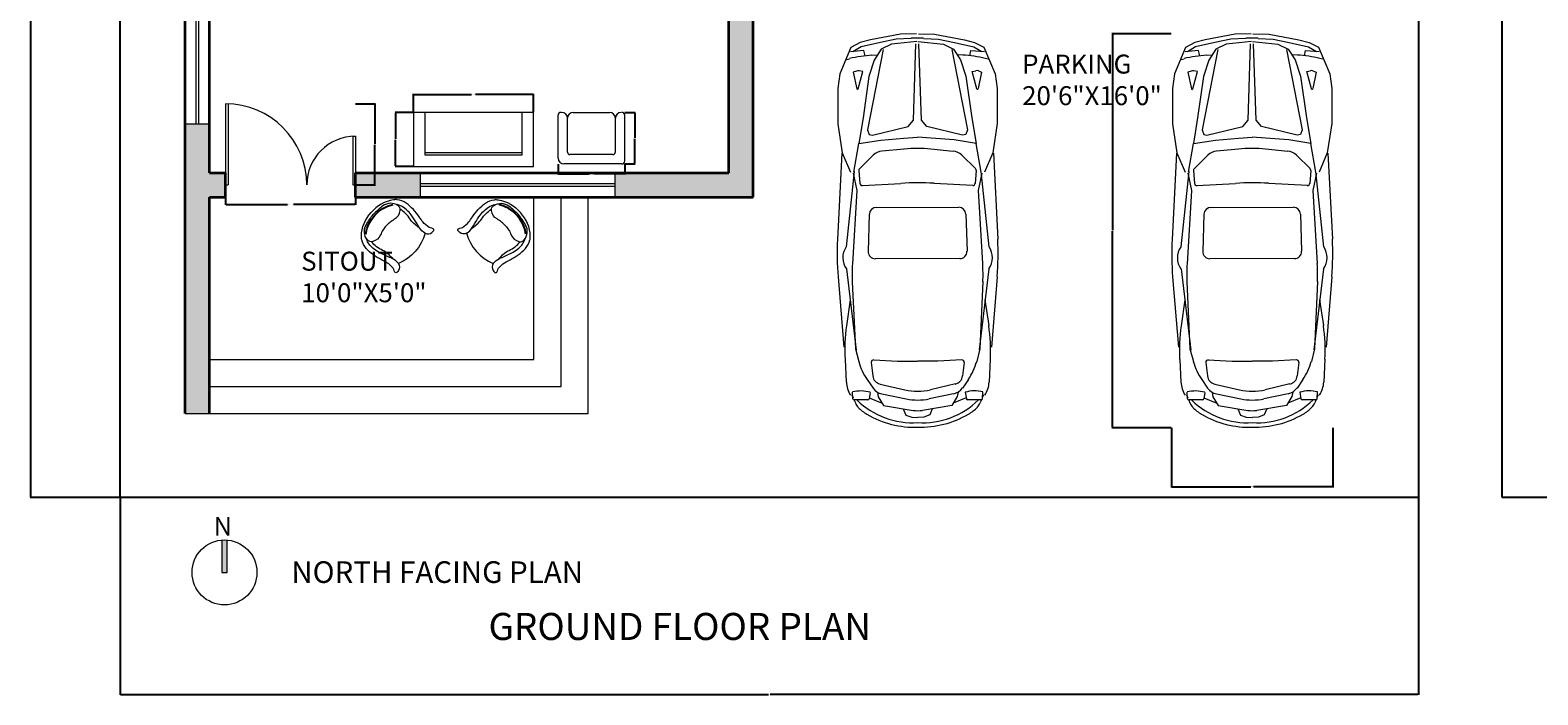
# Model space of a CAD drawing. Units: inches. Extents: x 3386 to 4477, y 1118 to 1824.
# Tile 1 of 7: x 3386 to 3944, y 1118 to 1364. Entities that reach past the tile are written whole.
import ezdxf

# ---------------------------------------------------------------- set-up
doc = ezdxf.new("R2010")
doc.units = ezdxf.units.IN
for name, color, linetype, lineweight in [('A-ANNO-DIMS', 2, 'Continuous', 18), ('A-ANNO-SYMB', 7, 'Continuous', 18), ('A-ANNO-TITL', 7, 'Continuous', 25), ('A-AREA-IDEN', 7, 'Continuous', 18), ('A-DOOR', 4, 'Continuous', 18), ('A-FLOR-STRS', 7, 'Continuous', 18), ('A-FURN', 8, 'Continuous', 18), ('A-GLAZ', 4, 'Continuous', 18), ('A-SITE-VEHI', 8, 'Continuous', 13), ('A-WALL', 7, 'Continuous', 35), ('C-PROP', 7, 'Continuous', 25)]:
    doc.layers.add(name, color=color, linetype=linetype, lineweight=lineweight)
doc.layers.add('A-WALL-PATT', color=18, linetype='Continuous', lineweight=13, true_color=0x000000)
doc.layers.add('IFF-FURN-DETAIL', color=250, linetype='Continuous')
doc.styles.get("Standard").update_dxf_attribs({"font": 'arial.ttf'})
doc.dimstyles.get("Standard").update_dxf_attribs({"dimtxt": 0.18, "dimasz": 0.18, "dimexe": 0.18, "dimexo": 0.0625, "dimgap": 0.09, "dimtad": 0, "dimtih": 1, "dimtoh": 1, "dimdec": 4, "dimzin": 0, "dimdsep": 46, "dimtxsty": 'Standard', "dimcen": 0.09, "dimadec": 0, "dimazin": 0, "dimtfac": 1, "dimtdec": 4, "dimtofl": 0, "dimtmove": 0, "dimatfit": 3, "dimfxl": 1, "dimtolj": 1, "dimtzin": 0, "dimarcsym": 0})

# ---------------------------------------------------------------- blocks, each defined once
blk = doc.blocks.new('D')
for p, q in [((0, 30), (0, 0)), ((1, 29.93), (1, 0)), ((47, 18), (47, 0)), ((47, 18), (48, 18)), ((48, 18), (48, 0)), ((0, 0), (1, 0)), ((47, 0), (48, 0))]:
    blk.add_line(p, q)
for centre, radius, start, end in [((0, 0), 30, 0, 90), ((48, 0), 18, 90, 180)]:
    blk.add_arc(centre, radius, start, end)
blk = doc.blocks.new('sofa-27')
at = {"color": 0, "linetype": 'ByBlock'}
for p, q in [((-0.059, 0.059), (-0.059, 0.49)), ((0.035, 0.118), (0.035, 0.461)), ((0.094, 0.52), (0.459, 0.52)), ((0.518, 0.118), (0.518, 0.461)), ((0.613, 0.03), (0.613, 0.49)), ((0.583, 0), (0, 0)), ((0.494, 0.094), (0.059, 0.094))]:
    blk.add_line(p, q, dxfattribs=at)
for centre, radius, start, end in [((-0.03, 0.49), 0.0295, 90, 180), ((-0.024, 0.461), 0.0591, 360, 90), ((0.094, 0.461), 0.0591, 90, 180), ((0.459, 0.461), 0.0591, 0, 90), ((0.577, 0.461), 0.0591, 90, 180), ((0.583, 0.49), 0.0295, 0, 90), ((0, 0.059), 0.0591, 180, 270), ((0.059, 0.118), 0.0236, 180, 270), ((0.494, 0.118), 0.0236, 270, 0), ((0.583, 0.03), 0.0295, 270, 0)]:
    blk.add_arc(centre, radius, start, end, dxfattribs=at)
blk = doc.blocks.new('12PCOU24')
for p, q in [((9.6, 33.9), (9.6, -34.1)), ((38, 33.9), (38, -34.1))]:
    blk.add_line(p, q)
blk.add_lwpolyline([(0, 42.1), (38, 42.1), (38, 33.9), (8, 33.9), (8, -34.1), (38, -34.1), (38, -42.1), (0, -42.1)], close=True)
blk = doc.blocks.new('A$C4A3239E3')
for p, q in [((1.251, 1.634), (2.152, 1.68)), ((1.443, 1.502), (2.231, 1.588)), ((2.463, 1.587), (3.312, 1.486)), ((2.545, 1.674), (3.282, 1.615)), ((2.788, 1.546), (3.057, 1.586)), ((3.41, 1.602), (3.649, 1.59)), ((0.09, 1.227), (0.136, 1.429)), ((0.136, 1.429), (0.187, 1.515)), ((0.175, 1.399), (0.187, 1.541)), ((0.266, 1.579), (0.259, 1.549)), ((0.396, 1.412), (0.388, 1.449)), ((0.39, 1.477), (0.402, 1.511)), ((0.576, 1.46), (0.396, 1.412)), ((0.402, 1.511), (0.575, 1.474)), ((1.45, 1.506), (1.149, 1.455)), ((1.272, 1.303), (1.413, 1.446)), ((1.433, 1.454), (1.567, 1.444)), ((1.461, 1.515), (1.641, 1.474)), ((1.641, 1.474), (2.408, 1.522)), ((2.597, 1.524), (3.301, 1.494)), ((3.301, 1.494), (3.432, 1.46)), ((3.822, 1.52), (3.752, 1.525)), ((3.781, 1.532), (3.813, 1.518)), ((3.833, 1.363), (3.833, 1.508)), ((3.838, 1.508), (3.867, 1.496)), ((0.231, 1.387), (0.175, 1.399)), ((0.224, 1.314), (0.221, 1.265)), ((1.59, 1.418), (1.567, 1.013)), ((1.819, 0.408), (1.818, 1.271)), ((1.89, 1.345), (2.279, 1.358)), ((2.356, 1.283), (2.357, 0.397)), ((3.416, 1.302), (3.429, 1.052)), ((3.443, 1.328), (3.584, 1.312)), ((3.622, 1.372), (3.711, 1.31)), ((3.753, 1.264), (3.801, 1.255)), ((3.756, 1.339), (3.823, 1.351)), ((3.814, 1.35), (3.869, 1.214)), ((0.056, 1.059), (0.09, 1.227)), ((1.207, 0.98), (1.229, 1.212)), ((3.669, 1.236), (3.73, 0.976)), ((3.771, 1.218), (3.825, 0.963)), ((3.801, 1.255), (3.894, 1.199)), ((3.894, 1.199), (3.945, 0.89)), ((0.048, 0.904), (0.056, 1.059)), ((3.429, 1.052), (3.429, 0.843)), ((3.929, 0.994), (3.993, 0.967)), ((3.993, 0.967), (4.017, 0.906)), ((3.43, 0.631), (3.429, 0.84)), ((3.895, 0.484), (3.945, 0.793)), ((4.017, 0.906), (4.021, 0.842)), ((4.017, 0.778), (4.021, 0.842)), ((0.048, 0.772), (0.057, 0.617)), ((1.208, 0.698), (1.23, 0.466)), ((1.591, 0.261), (1.567, 0.666)), ((3.67, 0.447), (3.73, 0.707)), ((3.772, 0.465), (3.825, 0.721)), ((3.929, 0.689), (3.994, 0.717)), ((3.994, 0.717), (4.017, 0.778)), ((0.057, 0.617), (0.091, 0.45)), ((3.417, 0.38), (3.43, 0.631)), ((3.802, 0.428), (3.895, 0.484)), ((0.091, 0.45), (0.137, 0.247)), ((0.225, 0.362), (0.222, 0.411)), ((1.273, 0.375), (1.415, 0.232)), ((1.891, 0.334), (2.28, 0.323)), ((3.444, 0.354), (3.585, 0.371)), ((3.623, 0.311), (3.712, 0.373)), ((3.754, 0.419), (3.802, 0.428)), ((3.757, 0.344), (3.824, 0.333)), ((3.815, 0.333), (3.869, 0.469)), ((3.834, 0.32), (3.835, 0.175)), ((0.137, 0.247), (0.188, 0.161)), ((0.232, 0.29), (0.176, 0.277)), ((0.176, 0.277), (0.188, 0.136)), ((0.397, 0.265), (0.389, 0.228)), ((0.391, 0.2), (0.403, 0.166)), ((0.577, 0.217), (0.397, 0.265)), ((0.403, 0.166), (0.577, 0.203)), ((1.451, 0.172), (1.15, 0.223)), ((1.434, 0.225), (1.568, 0.235)), ((1.444, 0.176), (2.233, 0.092)), ((1.462, 0.164), (1.642, 0.205)), ((1.642, 0.205), (2.409, 0.158)), ((2.464, 0.094), (3.313, 0.196)), ((2.598, 0.156), (3.302, 0.188)), ((3.302, 0.188), (3.433, 0.223)), ((3.823, 0.163), (3.753, 0.158)), ((3.783, 0.151), (3.814, 0.165)), ((3.839, 0.175), (3.868, 0.188)), ((0.268, 0.097), (0.261, 0.127)), ((1.252, 0.045), (2.154, 0)), ((2.546, 0.006), (3.283, 0.067)), ((2.789, 0.135), (3.058, 0.096)), ((3.412, 0.08), (3.651, 0.093))]:
    blk.add_line(p, q)
for points in [[(0, 0.848), (0.005, 1.016), (0.062, 1.33), (0.09, 1.438), (0.141, 1.536), (0.419, 1.653), (0.572, 1.674), (0.94, 1.674), (1.246, 1.627), (1.45, 1.541)], [(0.081, 0.844), (0.109, 1.11), (0.161, 1.218), (0.274, 1.291), (0.446, 1.347), (0.881, 1.409), (1.149, 1.455), (1.112, 1.224), (1.093, 0.981), (1.085, 0.839)], [(0.164, 1.198), (1.007, 1.364), (1.054, 1.346), (1.062, 1.312), (0.971, 0.937), (0.904, 0.882), (0.106, 0.853)], [(0, 0.828), (0.006, 0.66), (0.063, 0.346), (0.092, 0.239), (0.143, 0.14), (0.42, 0.024), (0.574, 0.003), (0.942, 0.003), (1.247, 0.051), (1.451, 0.138)], [(0.081, 0.832), (0.109, 0.566), (0.162, 0.458), (0.275, 0.386), (0.447, 0.33), (0.882, 0.268), (1.15, 0.223), (1.113, 0.454), (1.094, 0.696), (1.085, 0.839)], [(0.165, 0.478), (1.008, 0.314), (1.055, 0.332), (1.063, 0.366), (0.971, 0.741), (0.904, 0.796), (0.106, 0.823)]]:
    blk.add_lwpolyline(points)
for centre, radius, start, end in [((2.305, -1.296), 2.98, 85.3952, 92.9452), ((2.346, 1.423), 0.202, 54.6492, 124.7769), ((3.317, -0.183), 1.788, 86.9998, 98.3676), ((3.635, 1.312), 0.278, 57.3299, 87.1824), ((1.71, 1.212), 1.49, 166.9166, 176.0811), ((0.436, 1.46), 0.0497, 159.9787, 192.5384), ((0.574, 1.467), 0.00745, 284.96, 78.1125), ((1.431, 1.429), 0.0248, 85.7151, 135.3046), ((1.565, 1.419), 0.0248, 356.7256, 85.7151), ((2.521, -0.262), 1.788, 87.5491, 93.6237), ((3.28, 0.883), 0.596, 55.07, 75.2551), ((4.097, 1.439), 0.356, 166.0961, 196.3535), ((3.821, 1.508), 0.0124, 0, 86.3304), ((3.247, 0.896), 0.828, 356.2451, 44.5195), ((3.809, 1.358), 0.149, 46.3836, 67.2014), ((3.618, 1.158), 0.426, 30.4577, 46.3836), ((1.378, 1.198), 0.149, 135.3046, 174.6214), ((1.892, 1.271), 0.0745, 91.8201, 179.9989), ((2.281, 1.283), 0.0745, 359.9245, 91.8201), ((3.441, 1.304), 0.0248, 83.376, 183.115), ((3.573, 1.213), 0.0993, 13.1226, 83.376), ((3.625, 1.188), 0.149, 11.7694, 55.07), ((3.821, 1.363), 0.0124, 279.6077, 0), ((3.132, 0.872), 0.989, 358.0694, 30.4577), ((2.691, 0.84), 1.49, 174.6214, 185.4916), ((4.542, 0.842), 2.98, 176.7256, 183.3874), ((3.149, 0.841), 0.596, 346.9903, 13.1226), ((3.241, 0.841), 0.596, 348.3436, 11.7694), ((1.238, 0.839), 1.192, 176.8942, 183.2188), ((3.247, 0.786), 0.828, 315.5935, 3.8679), ((3.651, 0.841), 0.298, 350.7246, 9.3883), ((3.133, 0.809), 0.989, 329.6553, 2.0435), ((1.711, 0.467), 1.49, 184.0319, 193.1964), ((1.378, 0.48), 0.149, 185.4916, 224.8083), ((1.893, 0.409), 0.0745, 180.1141, 268.2929), ((2.282, 0.397), 0.0745, 268.2929, 0.1885), ((3.441, 0.379), 0.0248, 176.9979, 276.737), ((3.573, 0.469), 0.0993, 276.737, 346.9903), ((3.626, 0.495), 0.149, 305.0429, 348.3436), ((4.098, 0.244), 0.356, 163.7595, 194.0169), ((3.822, 0.32), 0.0124, 0.113, 80.5053), ((0.438, 0.217), 0.0497, 167.5746, 200.1342), ((0.575, 0.21), 0.00745, 282.0005, 75.153), ((1.432, 0.249), 0.0248, 224.8083, 274.3979), ((1.566, 0.26), 0.0248, 274.3979, 3.3874), ((3.281, 0.799), 0.596, 284.8579, 305.0429), ((3.822, 0.175), 0.0124, 273.7825, 0.113), ((3.81, 0.325), 0.149, 292.9116, 313.7293), ((3.619, 0.525), 0.426, 313.7293, 329.6553), ((2.301, 2.976), 2.98, 267.1678, 274.7177), ((2.347, 0.258), 0.202, 235.336, 305.4638), ((2.518, 1.942), 1.788, 266.4893, 272.5638), ((3.315, 1.865), 1.788, 261.7454, 273.1132), ((3.636, 0.371), 0.278, 272.9306, 302.783)]:
    blk.add_arc(centre, radius, start, end)
blk = doc.blocks.new('ILNG95')
for points in [[(120, 308, -0.32971), (51, 384, -0.036099), (50, 422, -0.497733), (75, 439, -0.070621), (96, 429, 0.101868), (133, 414, 0.091794), (259, 412, 0.024114), (351, 433, -0.090294), (638, 458, -0.132412), (775, 407, -0.068618), (816, 368, -0.184346), (943, 0, 1.803905)], [(120, 308, 0.138132), (244, 313, 0.001085), (325, 339, -0.034227), (462, 375, -0.033255), (567, 387, -0.137428), (727, 350, -4.561553)], [(120, 308, 0.138132), (244, 313, 0.001085), (325, 339, -0.034227), (462, 375, -0.033255), (567, 387, -0.137428), (727, 350, -4.561553)], [(235, 308, 0.064243), (394, 307, 0.04414), (433, 315, -0.118032), (643, 329, -6.296816)], [(235, 308, 0.064243), (394, 307, 0.04414), (433, 315, -0.118032), (643, 329, -6.296816)], [(639, 0, 0.078302), (612, 161, -0.233633), (633, 315, -0.28763), (710, 349, -0.317923), (875, 193, -0.032882), (900, 0, 1.140397)], [(639, 0, 0.078302), (612, 161, -0.233633), (633, 315, -0.28763), (710, 349, -0.317923), (875, 193, -0.032882), (900, 0, 1.140397)], [(120, -308, 0.32971), (51, -384, 0.036099), (50, -422, 0.497733), (75, -439, 0.070621), (96, -429, -0.101868), (133, -414, -0.091794), (259, -412, -0.024114), (351, -433, 0.090294), (638, -458, 0.132412), (775, -407, 0.068618), (816, -368, 0.184346), (943, 0, -1.803905)], [(639, 0, -0.078302), (612, -161, 0.233633), (633, -315, 0.28763), (710, -349, 0.317923), (875, -193, 0.032882), (900, 0, -1.140397)], [(639, 0, -0.078302), (612, -161, 0.233633), (633, -315, 0.28763), (710, -349, 0.317923), (875, -193, 0.032882), (900, 0, -1.140397)], [(120, -308, -0.138132), (244, -313, -0.001085), (325, -339, 0.034227), (462, -375, 0.033255), (567, -387, 0.137428), (727, -350, 4.561553)], [(120, -308, -0.138132), (244, -313, -0.001085), (325, -339, 0.034227), (462, -375, 0.033255), (567, -387, 0.137428), (727, -350, 4.561553)], [(235, -308, -0.064243), (394, -307, -0.04414), (433, -315, 0.118032), (643, -329, 6.296816)], [(235, -308, -0.064243), (394, -307, -0.04414), (433, -315, 0.118032), (643, -329, 6.296816)]]:
    blk.add_lwpolyline(points, format="xyb")
blk.add_arc((759, 1), 709, 154.3281, 205.801)
at = {"layer": 'IFF-FURN-DETAIL'}
blk.add_arc((326, -2), 549, 326.8997, 34.6691, dxfattribs=at)
blk.add_arc((326, -2), 549, 326.8997, 34.6691, dxfattribs=at)
blk = doc.blocks.new('WIN-48IN')
for p, q in [((0, 48), (9, 48)), ((4, 0), (4, 48)), ((5, 0), (5, 48)), ((0, 0), (9, 0))]:
    blk.add_line(p, q)
blk = doc.blocks.new('WIN-72IN')
for p, q in [((0, 0), (0, 9)), ((72, 0), (72, 9)), ((0, 5), (72, 5)), ((0, 4), (72, 4))]:
    blk.add_line(p, q)
blk = doc.blocks.new('NORTH-ARROW')
at = {"transparency": 33554687}
h = blk.add_hatch(color=256, dxfattribs=at)
h.dxf.hatch_style = 1
h.paths.add_polyline_path([(1, 0), (-1, 0), (-1, 11.96, -0.020861), (0, 12, -0.020861), (1, 11.96)])
for p, q in [((-1, 12), (-1, 0)), ((1, 0), (1, 11.96)), ((-1, 0), (1, 0))]:
    blk.add_line(p, q)
blk.add_circle((0, 0), 12)
blk.add_text('N', height=6.9).set_placement((-4.02, 13.6))
blk = doc.blocks.new('*D63')
at = {"layer": 'A-ANNO-DIMS', "color": 0, "lineweight": -2, "transparency": 16777216}
for p, q in [((3458.66, 1306.31), (3458.66, 1298.99)), ((3506.66, 1306.31), (3506.66, 1298.99)), ((3458.84, 1299.17), (3481.57, 1299.17)), ((3506.48, 1299.17), (3483.74, 1299.17))]:
    blk.add_line(p, q, dxfattribs=at)
at = {"layer": 'A-ANNO-DIMS', "color": 0, "transparency": 16777216}
for points in [[(3458.84, 1299.2), (3458.84, 1299.14), (3458.66, 1299.17)], [(3506.48, 1299.2), (3506.48, 1299.14), (3506.66, 1299.17)]]:
    blk.add_solid(points, dxfattribs=at)
at = {"layer": 'Defpoints', "color": 0, "transparency": 16777216}
for p in [(3458.66, 1306.37), (3506.66, 1306.37), (3506.66, 1299.17)]:
    blk.add_point(p, dxfattribs=at)
at = {"layer": 'A-ANNO-DIMS', "color": 0, "transparency": 16777216, "insert": (3482.66, 1299.17), "char_height": 0.18, "attachment_point": 5}
blk.add_mtext('\\A1;ENTRY DOOR 48', dxfattribs=at)
blk = doc.blocks.new('*D64')
at = {"layer": 'A-ANNO-DIMS', "color": 0, "lineweight": -2, "transparency": 16777216}
for p, q in [((3506.72, 1336.37), (3514.04, 1336.37)), ((3513.86, 1336.19), (3513.86, 1321.55)), ((3513.86, 1306.55), (3513.86, 1321.19)), ((3506.72, 1306.37), (3514.04, 1306.37))]:
    blk.add_line(p, q, dxfattribs=at)
at = {"layer": 'A-ANNO-DIMS', "color": 0, "transparency": 16777216}
for points in [[(3513.83, 1336.19), (3513.89, 1336.19), (3513.86, 1336.37)], [(3513.83, 1306.55), (3513.89, 1306.55), (3513.86, 1306.37)]]:
    blk.add_solid(points, dxfattribs=at)
at = {"layer": 'Defpoints', "color": 0, "transparency": 16777216}
for p in [(3506.66, 1336.37), (3513.86, 1336.37), (3506.66, 1306.37)]:
    blk.add_point(p, dxfattribs=at)
at = {"layer": 'A-ANNO-DIMS', "color": 0, "transparency": 16777216, "insert": (3513.86, 1321.37), "char_height": 0.18, "attachment_point": 5}
blk.add_mtext('\\A1;30', dxfattribs=at)
blk = doc.blocks.new('*D71')
at = {"layer": 'A-ANNO-DIMS', "color": 0, "lineweight": -2, "transparency": 16777216}
for p, q in [((3581.59, 1314.07), (3581.59, 1310.26)), ((3581.77, 1310.44), (3593.01, 1310.44)), ((3606.03, 1310.44), (3594.79, 1310.44)), ((3606.21, 1314.07), (3606.21, 1310.26))]:
    blk.add_line(p, q, dxfattribs=at)
at = {"layer": 'A-ANNO-DIMS', "color": 0, "transparency": 16777216}
for points in [[(3581.77, 1310.47), (3581.77, 1310.41), (3581.59, 1310.44)], [(3606.03, 1310.47), (3606.03, 1310.41), (3606.21, 1310.44)]]:
    blk.add_solid(points, dxfattribs=at)
at = {"layer": 'Defpoints', "color": 0, "transparency": 16777216}
for p in [(3581.59, 1314.14), (3606.21, 1314.14), (3606.21, 1310.44)]:
    blk.add_point(p, dxfattribs=at)
at = {"layer": 'A-ANNO-DIMS', "color": 0, "transparency": 16777216, "insert": (3593.9, 1310.44), "char_height": 0.18, "attachment_point": 5}
blk.add_mtext('\\A1;SEAT 25 TYP.', dxfattribs=at)
blk = doc.blocks.new('*D72')
at = {"layer": 'A-ANNO-DIMS', "color": 0, "lineweight": -2, "transparency": 16777216}
for p, q in [((3606.28, 1333.19), (3610.09, 1333.19)), ((3609.91, 1333.01), (3609.91, 1323.85)), ((3609.91, 1314.32), (3609.91, 1323.48)), ((3606.28, 1314.14), (3610.09, 1314.14))]:
    blk.add_line(p, q, dxfattribs=at)
at = {"layer": 'A-ANNO-DIMS', "color": 0, "transparency": 16777216}
for points in [[(3609.88, 1333.01), (3609.94, 1333.01), (3609.91, 1333.19)], [(3609.88, 1314.32), (3609.94, 1314.32), (3609.91, 1314.14)]]:
    blk.add_solid(points, dxfattribs=at)
at = {"layer": 'Defpoints', "color": 0, "transparency": 16777216}
for p in [(3606.21, 1333.19), (3609.91, 1333.19), (3606.21, 1314.14)]:
    blk.add_point(p, dxfattribs=at)
at = {"layer": 'A-ANNO-DIMS', "color": 0, "transparency": 16777216, "insert": (3609.91, 1323.66), "char_height": 0.18, "attachment_point": 5}
blk.add_mtext('\\A1;19 TYP.', dxfattribs=at)
blk = doc.blocks.new('*D85')
at = {"layer": 'A-ANNO-DIMS', "color": 0, "lineweight": -2, "transparency": 16777216}
for p, q in [((3808.27, 1362.25), (3786.31, 1362.25)), ((3786.49, 1362.07), (3786.49, 1289.63)), ((3786.49, 1216.82), (3786.49, 1289.26)), ((3808.27, 1216.64), (3786.31, 1216.64))]:
    blk.add_line(p, q, dxfattribs=at)
at = {"layer": 'A-ANNO-DIMS', "color": 0, "transparency": 16777216}
for points in [[(3786.46, 1362.07), (3786.52, 1362.07), (3786.49, 1362.25)], [(3786.46, 1216.82), (3786.52, 1216.82), (3786.49, 1216.64)]]:
    blk.add_solid(points, dxfattribs=at)
at = {"layer": 'Defpoints', "color": 0, "transparency": 16777216}
for p in [(3808.33, 1362.25), (3786.49, 1216.64), (3808.33, 1216.64)]:
    blk.add_point(p, dxfattribs=at)
at = {"layer": 'A-ANNO-DIMS', "color": 0, "transparency": 16777216, "insert": (3786.49, 1289.45), "char_height": 0.18, "attachment_point": 5}
blk.add_mtext('\\A1;CAR 146 TYP.', dxfattribs=at)
blk = doc.blocks.new('*D86')
at = {"layer": 'A-ANNO-DIMS', "color": 0, "lineweight": -2, "transparency": 16777216}
for p, q in [((3808.33, 1216.58), (3808.33, 1194.62)), ((3868.05, 1216.58), (3868.05, 1194.62)), ((3808.51, 1194.8), (3837.66, 1194.8)), ((3867.87, 1194.8), (3838.72, 1194.8))]:
    blk.add_line(p, q, dxfattribs=at)
at = {"layer": 'A-ANNO-DIMS', "color": 0, "transparency": 16777216}
for points in [[(3808.51, 1194.83), (3808.51, 1194.77), (3808.33, 1194.8)], [(3867.87, 1194.83), (3867.87, 1194.77), (3868.05, 1194.8)]]:
    blk.add_solid(points, dxfattribs=at)
at = {"layer": 'Defpoints', "color": 0, "transparency": 16777216}
for p in [(3808.33, 1216.64), (3868.05, 1216.64), (3868.05, 1194.8)]:
    blk.add_point(p, dxfattribs=at)
at = {"layer": 'A-ANNO-DIMS', "color": 0, "transparency": 16777216, "insert": (3838.19, 1194.8), "char_height": 0.18, "attachment_point": 5}
blk.add_mtext('\\A1;60 TYP.', dxfattribs=at)
blk = doc.blocks.new('*D93')
at = {"layer": 'A-ANNO-DIMS', "color": 0, "lineweight": -2, "transparency": 16777216}
for p, q in [((3528.17, 1333.25), (3528.17, 1340.01)), ((3528.35, 1339.83), (3549.62, 1339.83)), ((3572.27, 1339.83), (3551, 1339.83)), ((3572.45, 1333.25), (3572.45, 1340.01))]:
    blk.add_line(p, q, dxfattribs=at)
at = {"layer": 'A-ANNO-DIMS', "color": 0, "transparency": 16777216}
for points in [[(3528.35, 1339.86), (3528.35, 1339.8), (3528.17, 1339.83)], [(3572.27, 1339.86), (3572.27, 1339.8), (3572.45, 1339.83)]]:
    blk.add_solid(points, dxfattribs=at)
at = {"layer": 'Defpoints', "color": 0, "transparency": 16777216}
for p in [(3572.45, 1339.83), (3528.17, 1333.19), (3572.45, 1333.19)]:
    blk.add_point(p, dxfattribs=at)
at = {"layer": 'A-ANNO-DIMS', "color": 0, "transparency": 16777216, "insert": (3550.31, 1339.83), "char_height": 0.18, "attachment_point": 5}
blk.add_mtext('\\A1;BENCH 44', dxfattribs=at)
blk = doc.blocks.new('*D94')
at = {"layer": 'A-ANNO-DIMS', "color": 0, "lineweight": -2, "transparency": 16777216}
for p, q in [((3528.11, 1333.19), (3521.35, 1333.19)), ((3521.53, 1333.01), (3521.53, 1323.39)), ((3521.53, 1313.4), (3521.53, 1323.02)), ((3528.11, 1313.22), (3521.35, 1313.22))]:
    blk.add_line(p, q, dxfattribs=at)
at = {"layer": 'A-ANNO-DIMS', "color": 0, "transparency": 16777216}
for points in [[(3521.5, 1333.01), (3521.56, 1333.01), (3521.53, 1333.19)], [(3521.5, 1313.4), (3521.56, 1313.4), (3521.53, 1313.22)]]:
    blk.add_solid(points, dxfattribs=at)
at = {"layer": 'Defpoints', "color": 0, "transparency": 16777216}
for p in [(3521.53, 1333.19), (3528.17, 1333.19), (3528.17, 1313.22)]:
    blk.add_point(p, dxfattribs=at)
at = {"layer": 'A-ANNO-DIMS', "color": 0, "transparency": 16777216, "insert": (3521.53, 1323.2), "char_height": 0.18, "attachment_point": 5}
blk.add_mtext('\\A1;20', dxfattribs=at)
blk = doc.blocks.new('*D101')
at = {"layer": 'A-ANNO-DIMS', "color": 0, "lineweight": -2, "transparency": 16777216}
for p, q in [((3419.66, 1190.81), (3419.66, 1117.96)), ((3899.66, 1190.81), (3899.66, 1117.96)), ((3419.84, 1118.14), (3659.36, 1118.14)), ((3899.48, 1118.14), (3659.95, 1118.14))]:
    blk.add_line(p, q, dxfattribs=at)
at = {"layer": 'A-ANNO-DIMS', "color": 0, "transparency": 16777216}
for points in [[(3419.84, 1118.17), (3419.84, 1118.11), (3419.66, 1118.14)], [(3899.48, 1118.17), (3899.48, 1118.11), (3899.66, 1118.14)]]:
    blk.add_solid(points, dxfattribs=at)
at = {"layer": 'Defpoints', "color": 0, "transparency": 16777216}
for p in [(3419.66, 1190.87), (3899.66, 1190.87), (3899.66, 1118.14)]:
    blk.add_point(p, dxfattribs=at)
at = {"layer": 'A-ANNO-DIMS', "color": 0, "transparency": 16777216, "insert": (3659.66, 1118.14), "char_height": 0.18, "attachment_point": 5}
blk.add_mtext('\\A1;480', dxfattribs=at)
blk = doc.blocks.new('*D102')
at = {"layer": 'A-ANNO-DIMS', "color": 0, "lineweight": -2, "transparency": 16777216}
for p, q in [((3419.59, 1790.87), (3386.43, 1790.87)), ((3386.61, 1790.69), (3386.61, 1491.05)), ((3386.61, 1191.05), (3386.61, 1490.69)), ((3419.59, 1190.87), (3386.43, 1190.87))]:
    blk.add_line(p, q, dxfattribs=at)
at = {"layer": 'A-ANNO-DIMS', "color": 0, "transparency": 16777216}
for points in [[(3386.58, 1790.69), (3386.64, 1790.69), (3386.61, 1790.87)], [(3386.58, 1191.05), (3386.64, 1191.05), (3386.61, 1190.87)]]:
    blk.add_solid(points, dxfattribs=at)
at = {"layer": 'Defpoints', "color": 0, "transparency": 16777216}
for p in [(3386.61, 1790.87), (3419.66, 1790.87), (3419.66, 1190.87)]:
    blk.add_point(p, dxfattribs=at)
at = {"layer": 'A-ANNO-DIMS', "color": 0, "transparency": 16777216, "insert": (3386.61, 1490.87), "char_height": 0.18, "attachment_point": 5}
blk.add_mtext('\\A1;600', dxfattribs=at)
blk = doc.blocks.new('*D106')
at = {"layer": 'A-ANNO-DIMS', "color": 0, "lineweight": -2, "transparency": 16777216}
for p, q in [((3963.65, 1790.87), (3930.48, 1790.87)), ((3930.66, 1790.69), (3930.66, 1491.05)), ((3930.66, 1191.05), (3930.66, 1490.69)), ((3963.65, 1190.87), (3930.48, 1190.87))]:
    blk.add_line(p, q, dxfattribs=at)
at = {"layer": 'A-ANNO-DIMS', "color": 0, "transparency": 16777216}
for points in [[(3930.63, 1790.69), (3930.69, 1790.69), (3930.66, 1790.87)], [(3930.63, 1191.05), (3930.69, 1191.05), (3930.66, 1190.87)]]:
    blk.add_solid(points, dxfattribs=at)
at = {"layer": 'Defpoints', "color": 0, "transparency": 16777216}
for p in [(3930.66, 1790.87), (3963.71, 1790.87), (3963.71, 1190.87)]:
    blk.add_point(p, dxfattribs=at)
at = {"layer": 'A-ANNO-DIMS', "color": 0, "transparency": 16777216, "insert": (3930.66, 1490.87), "char_height": 0.18, "attachment_point": 5}
blk.add_mtext('\\A1;600', dxfattribs=at)

msp = doc.modelspace()

# ---------------------------------------------------------------- hatches: boundary and pattern name
at = {"layer": 'A-WALL-PATT'}
h = msp.add_hatch(color=256, dxfattribs=at)
h.dxf.hatch_style = 1
h.paths.add_polyline_path([(3443.66, 1221.87), (3452.66, 1221.87), (3452.66, 1301.87), (3458.66, 1301.87), (3458.66, 1310.87), (3452.66, 1310.87), (3452.66, 1328.87), (3443.66, 1328.87)])
h.paths.add_polyline_path([(3506.66, 1310.87), (3506.66, 1306.37), (3506.66, 1301.87), (3530.66, 1301.87), (3530.66, 1310.87)])
h.paths.add_polyline_path([(3653.66, 1301.87), (3653.66, 1382.87), (3662.66, 1382.87), (3662.66, 1391.87), (3653.66, 1391.87), (3653.66, 1529.87), (3659.66, 1529.87), (3659.66, 1535.87), (3644.66, 1535.87), (3644.66, 1310.87), (3602.66, 1310.87), (3602.66, 1301.87)])
h.paths.add_polyline_path([(3452.66, 1406.87), (3443.66, 1406.87), (3443.66, 1376.87), (3452.66, 1376.87), (3452.66, 1388.44)])
h.paths.add_polyline_path([(3452.66, 1478.87), (3452.66, 1502.87), (3478.74, 1502.87), (3482.66, 1502.87), (3482.66, 1504.87), (3482.66, 1517.87), (3473.66, 1517.87), (3473.66, 1511.87), (3443.66, 1511.87), (3443.66, 1478.87)])
h.paths.add_polyline_path([(3773.66, 1391.87), (3710.66, 1391.87), (3710.66, 1382.87), (3773.66, 1382.87)], flags=17)
h.paths.add_polyline_path([(3824.66, 1391.87), (3806.66, 1391.87), (3806.66, 1469.87), (3809.66, 1469.87), (3809.66, 1472.87), (3809.66, 1475.87), (3806.66, 1475.87), (3806.66, 1478.87), (3800.66, 1478.87), (3800.66, 1463.32), (3800.66, 1391.87), (3797.66, 1391.87), (3797.66, 1382.87), (3824.66, 1382.87)], flags=17)
h.paths.add_polyline_path([(3866.66, 1469.87), (3866.66, 1391.87), (3848.66, 1391.87), (3848.66, 1382.87), (3875.66, 1382.87), (3875.66, 1547.87), (3866.66, 1547.87), (3866.66, 1535.87), (3695.66, 1535.87), (3695.66, 1529.87), (3800.66, 1529.87), (3800.66, 1508.87), (3806.66, 1508.87), (3806.66, 1529.87), (3866.66, 1529.87), (3866.66, 1475.87), (3839.66, 1475.87), (3839.66, 1469.87)])
h.paths.add_polyline_path([(3875.66, 1673.87), (3866.66, 1673.87), (3866.66, 1663.37), (3866.66, 1647.44), (3866.66, 1613.87), (3761.66, 1613.87), (3761.66, 1607.87), (3866.66, 1607.87), (3866.66, 1595.87), (3875.66, 1595.87)])
h.paths.add_polyline_path([(3473.66, 1607.87), (3473.66, 1601.87), (3482.66, 1601.87), (3482.66, 1616.87), (3452.66, 1616.87), (3452.66, 1640.87), (3443.66, 1640.87), (3443.66, 1607.87)])
h.paths.add_polyline_path([(3491.66, 1736.87), (3491.66, 1745.87), (3478.95, 1745.87), (3443.66, 1745.87), (3443.66, 1688.87), (3452.66, 1688.87), (3452.66, 1736.87)])
h.paths.add_polyline_path([(3551.66, 1745.87), (3539.66, 1745.87), (3539.66, 1736.87), (3551.66, 1736.87)])
h.paths.add_polyline_path([(3587.66, 1745.87), (3581.66, 1745.87), (3581.66, 1741.37), (3581.66, 1736.87), (3587.66, 1736.87), (3587.66, 1712.87), (3596.66, 1712.87), (3596.66, 1757.87), (3644.66, 1757.87), (3644.66, 1679.87), (3596.66, 1679.87), (3596.66, 1682.87), (3592.16, 1682.87), (3587.66, 1682.87), (3587.66, 1607.87), (3602.66, 1607.87), (3602.66, 1613.87), (3596.66, 1613.87), (3596.66, 1673.87), (3644.66, 1673.87), (3644.66, 1613.87), (3638.66, 1613.87), (3638.66, 1610.87), (3638.66, 1607.87), (3725.66, 1607.87), (3725.66, 1613.87), (3722.66, 1613.87), (3722.66, 1634.87), (3716.66, 1634.87), (3716.66, 1613.87), (3650.66, 1613.87), (3650.66, 1673.87), (3683.66, 1673.87), (3683.66, 1679.87), (3650.66, 1679.87), (3650.66, 1757.87), (3671.66, 1757.87), (3671.66, 1766.87), (3587.66, 1766.87)])
h.paths.add_polyline_path([(3716.66, 1757.87), (3716.66, 1679.87), (3713.66, 1679.87), (3713.66, 1673.87), (3716.66, 1673.87), (3716.66, 1664.87), (3722.66, 1664.87), (3722.66, 1757.87), (3728.66, 1757.87), (3728.66, 1766.87), (3695.66, 1766.87), (3695.66, 1757.87)])
h.paths.add_polyline_path([(3806.66, 1757.87), (3806.66, 1766.87), (3776.66, 1766.87), (3776.66, 1757.87)])
h.paths.add_polyline_path([(3875.66, 1766.87), (3854.66, 1766.87), (3854.66, 1757.87), (3866.66, 1757.87), (3866.66, 1733.87), (3875.66, 1733.87)])

# ---------------------------------------------------------------- linework, layer by layer
at = {"layer": 'A-FLOR-STRS'}
for p, q in [((3572.66, 1241.87), (3572.66, 1301.87)), ((3582.66, 1231.87), (3582.66, 1301.87)), ((3592.66, 1221.87), (3592.66, 1301.87)), ((3452.66, 1241.87), (3572.66, 1241.87)), ((3452.66, 1231.87), (3582.66, 1231.87)), ((3443.66, 1221.87), (3592.66, 1221.87))]:
    msp.add_line(p, q, dxfattribs=at)
at = {"layer": 'A-WALL'}
for p, q in [((3644.66, 1310.87), (3644.66, 1535.87)), ((3443.66, 1221.87), (3443.66, 1511.87)), ((3452.66, 1310.87), (3452.66, 1502.87)), ((3653.66, 1301.87), (3653.66, 1382.87)), ((3452.66, 1310.87), (3458.66, 1310.87)), ((3458.66, 1301.87), (3458.66, 1310.87)), ((3506.66, 1301.87), (3506.66, 1310.87)), ((3506.66, 1310.87), (3644.66, 1310.87)), ((3452.66, 1221.87), (3452.66, 1301.87)), ((3452.66, 1301.87), (3458.66, 1301.87)), ((3506.66, 1301.87), (3653.66, 1301.87))]:
    msp.add_line(p, q, dxfattribs=at)
at = {"layer": 'C-PROP'}
msp.add_lwpolyline([(3419.66, 1790.87), (3899.66, 1790.87), (3899.66, 1190.87), (3419.66, 1190.87)], close=True, dxfattribs=at)

# ---------------------------------------------------------------- block references
at = {"layer": 'A-ANNO-SYMB'}
msp.add_blockref('NORTH-ARROW', (3458.24, 1163.19), dxfattribs=at)
at = {"layer": 'A-DOOR'}
msp.add_blockref('D', (3458.66, 1306.37), dxfattribs=at)
at = {"layer": 'A-FURN'}
for name, p, xscale, yscale, zscale, rotation in [('12PCOU24', (3550.31, 1313.22), -0.5256225248253119, 0.5256225248253119, 0.5256225248253119, 270), ('ILNG95', (3529.69, 1280.99), -0.0243705291132055, 0.0243705291132055, 0.0243705291132055, 318.5881218623716), ('ILNG95', (3550.45, 1280.99), 0.0243705291132055, 0.0243705291132055, 0.0243705291132055, 41.41187813762839)]:
    msp.add_blockref(name, p, dxfattribs=dict(at, xscale=xscale, yscale=yscale, zscale=zscale, rotation=rotation))
at = {"layer": 'A-FURN', "xscale": 36.66436083614781, "yscale": 36.66436083614781, "zscale": 36.66436083614781}
msp.add_blockref('sofa-27', (3583.76, 1314.14), dxfattribs=at)
at = {"layer": 'A-GLAZ', "rotation": 180}
msp.add_blockref('WIN-48IN', (3452.66, 1376.87), dxfattribs=at)
at = {"layer": 'A-GLAZ'}
msp.add_blockref('WIN-72IN', (3530.66, 1301.87), dxfattribs=at)
at = {"layer": 'A-SITE-VEHI', "xscale": 35.27598425228, "yscale": 35.27598425228, "zscale": 35.27598425228, "rotation": 270}
for p in [(3684.85, 1362.25), (3808.56, 1362.25)]:
    msp.add_blockref('A$C4A3239E3', p, dxfattribs=at)

# ---------------------------------------------------------------- texts
at = {"layer": 'A-ANNO-TITL', "attachment_point": 1}
for s, insert, char_height in [('{\\fTimes New Roman|b0|i0|c0|p18;NORTH FACING PLAN}', (3482.94, 1167.31), 8), ('{\\fTimes New Roman|b0|i0|c0|p18;GROUND FLOOR PLAN}', (3555.85, 1148.22), 10)]:
    msp.add_mtext_dynamic_manual_height_columns(s, width=196.2607, gutter_width=12.5, heights=[0], dxfattribs=dict(at, insert=insert, char_height=char_height))
at = {"layer": 'A-AREA-IDEN', "char_height": 7, "attachment_point": 1}
for s, insert in [('{\\fTimes New Roman|b0|i0|c0|p18;PARKING\\P20\'6"X16\'0"}', (3753.15, 1354.54)), ('{\\fTimes New Roman|b0|i0|c0|p18;SITOUT\\P10\'0"X5\'0"}', (3486.61, 1281.71))]:
    msp.add_mtext_dynamic_manual_height_columns(s, width=79.5604, gutter_width=12.5, heights=[0], dxfattribs=dict(at, insert=insert))

# ---------------------------------------------------------------- dimensions: what is measured, and where the dimension line sits
at = {"layer": 'A-ANNO-DIMS'}
for base, p1, p2, picture, middle in [((3386.61, 1790.87), (3419.66, 1190.87), (3419.66, 1790.87), '*D102', (3386.61, 1490.87)), ((3930.66, 1790.87), (3963.71, 1190.87), (3963.71, 1790.87), '*D106', (3930.66, 1490.87)), ((3513.86, 1336.37), (3506.66, 1306.37), (3506.66, 1336.37), '*D64', (3513.86, 1321.37)), ((3521.53, 1333.19), (3528.17, 1313.22), (3528.17, 1333.19), '*D94', (3521.53, 1323.2))]:
    dim = msp.add_linear_dim(base=base, p1=p1, p2=p2, angle=90, dimstyle='Standard', override={"dimdec": 0, "dimlfac": 1, "dimrnd": 0, "dimzin": 0, "dimdsep": 46, "dimlunit": 2}, dxfattribs=at)
    dim.commit()
    dim.dimension.update_dxf_attribs({"geometry": picture, "text_midpoint": middle})
for base, p1, p2, angle, text, picture, middle in [((3786.49, 1216.64), (3808.33, 1362.25), (3808.33, 1216.64), 270, 'CAR <> TYP.', '*D85', (3786.49, 1289.45)), ((3609.91, 1333.19), (3606.21, 1314.14), (3606.21, 1333.19), 90, '<> TYP.', '*D72', (3609.91, 1323.66))]:
    dim = msp.add_linear_dim(base=base, p1=p1, p2=p2, angle=angle, text=text, dimstyle='Standard', override={"dimdec": 0, "dimlfac": 1, "dimrnd": 0, "dimzin": 0, "dimdsep": 46, "dimlunit": 2}, dxfattribs=at)
    dim.commit()
    dim.dimension.update_dxf_attribs({"geometry": picture, "text_midpoint": middle})
for base, p1, p2, text, picture, middle in [((3572.45, 1339.83), (3528.17, 1333.19), (3572.45, 1333.19), 'BENCH <>', '*D93', (3550.31, 1339.83)), ((3606.21, 1310.44), (3581.59, 1314.14), (3606.21, 1314.14), 'SEAT <> TYP.', '*D71', (3593.9, 1310.44)), ((3506.66, 1299.17), (3458.66, 1306.37), (3506.66, 1306.37), 'ENTRY DOOR <>', '*D63', (3482.66, 1299.17)), ((3868.05, 1194.8), (3808.33, 1216.64), (3868.05, 1216.64), '<> TYP.', '*D86', (3838.19, 1194.8))]:
    dim = msp.add_linear_dim(base=base, p1=p1, p2=p2, text=text, dimstyle='Standard', override={"dimdec": 0, "dimlfac": 1, "dimrnd": 0, "dimzin": 0, "dimdsep": 46, "dimlunit": 2}, dxfattribs=at)
    dim.commit()
    dim.dimension.update_dxf_attribs({"geometry": picture, "text_midpoint": middle})
dim = msp.add_linear_dim(base=(3899.66, 1118.14), p1=(3419.66, 1190.87), p2=(3899.66, 1190.87), dimstyle='Standard', override={"dimdec": 0, "dimlfac": 1, "dimrnd": 0, "dimzin": 0, "dimdsep": 46, "dimlunit": 2}, dxfattribs=at)
dim.commit()
dim.dimension.update_dxf_attribs({"geometry": '*D101', "text_midpoint": (3659.66, 1118.14)})

doc.saveas('drawing.dxf')
